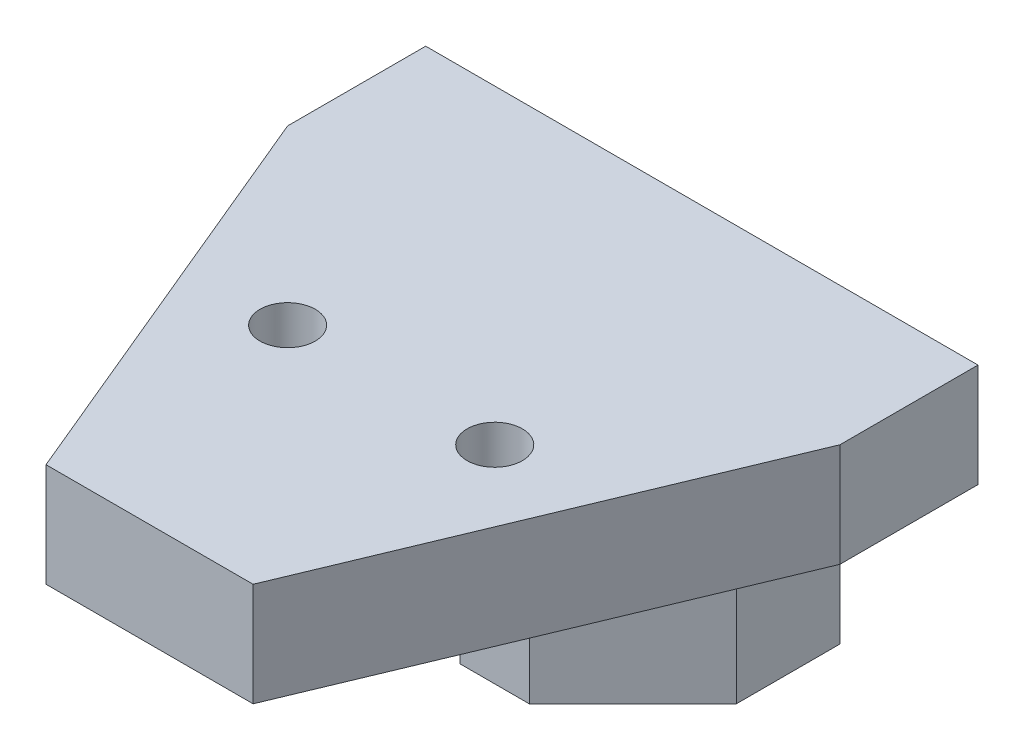
ISO-10303-21;
HEADER;
FILE_DESCRIPTION(('STEP AP214'),'2;1');
FILE_NAME('part.step','',(''),(''),'','','');
FILE_SCHEMA(('AUTOMOTIVE_DESIGN { 1 0 10303 214 1 1 1 1 }'));
ENDSEC;
DATA;
#1=APPLICATION_CONTEXT('core data for automotive mechanical design processes');
#2=APPLICATION_PROTOCOL_DEFINITION('international standard','automotive_design',2000,#1);
#3=PRODUCT_CONTEXT('',#1,'mechanical');
#4=PRODUCT('Part','Part','',(#3));
#5=PRODUCT_RELATED_PRODUCT_CATEGORY('part','',(#4));
#6=PRODUCT_DEFINITION_FORMATION('','',#4);
#7=PRODUCT_DEFINITION_CONTEXT('part definition',#1,'design');
#8=PRODUCT_DEFINITION('design','',#6,#7);
#9=PRODUCT_DEFINITION_SHAPE('','',#8);
#10=(LENGTH_UNIT() NAMED_UNIT(*) SI_UNIT(.MILLI.,.METRE.));
#11=(NAMED_UNIT(*) PLANE_ANGLE_UNIT() SI_UNIT($,.RADIAN.));
#12=(NAMED_UNIT(*) SI_UNIT($,.STERADIAN.) SOLID_ANGLE_UNIT());
#13=UNCERTAINTY_MEASURE_WITH_UNIT(LENGTH_MEASURE(1.E-05),#10,'distance_accuracy_value','');
#14=(GEOMETRIC_REPRESENTATION_CONTEXT(3) GLOBAL_UNCERTAINTY_ASSIGNED_CONTEXT((#13)) GLOBAL_UNIT_ASSIGNED_CONTEXT((#10,
#11,#12)) REPRESENTATION_CONTEXT('',''));
#15=CARTESIAN_POINT('',(0.,0.,0.));
#16=DIRECTION('',(0.,0.,1.));
#17=DIRECTION('',(1.,0.,0.));
#18=AXIS2_PLACEMENT_3D('',#15,#16,#17);
#19=CARTESIAN_POINT('',(0.,0.,20.));
#20=DIRECTION('',(0.,1.,0.));
#21=DIRECTION('',(0.,0.,1.));
#22=AXIS2_PLACEMENT_3D('',#19,#20,#21);
#23=PLANE('',#22);
#24=CARTESIAN_POINT('',(25.,0.,45.));
#25=DIRECTION('',(0.,-1.,0.));
#26=DIRECTION('',(0.,0.,-1.));
#27=AXIS2_PLACEMENT_3D('',#24,#25,#26);
#28=CIRCLE('',#27,4.);
#29=CARTESIAN_POINT('',(25.,0.,41.));
#30=VERTEX_POINT('',#29);
#31=EDGE_CURVE('E304',#30,#30,#28,.T.);
#32=ORIENTED_EDGE('',*,*,#31,.F.);
#33=EDGE_LOOP('',(#32));
#34=FACE_BOUND('',#33,.T.);
#35=CARTESIAN_POINT('',(55.,0.,45.));
#36=DIRECTION('',(0.,-1.,0.));
#37=DIRECTION('',(0.,0.,-1.));
#38=AXIS2_PLACEMENT_3D('',#35,#36,#37);
#39=CIRCLE('',#38,4.);
#40=CARTESIAN_POINT('',(55.,0.,41.));
#41=VERTEX_POINT('',#40);
#42=EDGE_CURVE('E305',#41,#41,#39,.T.);
#43=ORIENTED_EDGE('',*,*,#42,.F.);
#44=EDGE_LOOP('',(#43));
#45=FACE_BOUND('',#44,.T.);
#46=DIRECTION('',(0.,0.,-1.));
#47=VECTOR('',#46,1.);
#48=CARTESIAN_POINT('',(20.,0.,0.));
#49=LINE('',#48,#47);
#50=CARTESIAN_POINT('',(20.,0.,15.));
#51=VERTEX_POINT('',#50);
#52=CARTESIAN_POINT('',(20.,0.,0.));
#53=VERTEX_POINT('',#52);
#54=EDGE_CURVE('E58',#51,#53,#49,.T.);
#55=ORIENTED_EDGE('',*,*,#54,.F.);
#56=DIRECTION('',(-0.707106781186548,0.,-0.707106781186547));
#57=VECTOR('',#56,1.);
#58=CARTESIAN_POINT('',(35.,0.,30.));
#59=LINE('',#58,#57);
#60=CARTESIAN_POINT('',(35.,0.,30.));
#61=VERTEX_POINT('',#60);
#62=EDGE_CURVE('E64',#61,#51,#59,.T.);
#63=ORIENTED_EDGE('',*,*,#62,.F.);
#64=DIRECTION('',(-1.,0.,0.));
#65=VECTOR('',#64,1.);
#66=CARTESIAN_POINT('',(40.,0.,30.));
#67=LINE('',#66,#65);
#68=CARTESIAN_POINT('',(45.,0.,30.));
#69=VERTEX_POINT('',#68);
#70=EDGE_CURVE('E174',#69,#61,#67,.T.);
#71=ORIENTED_EDGE('',*,*,#70,.F.);
#72=DIRECTION('',(-0.707106781186547,0.,0.707106781186547));
#73=VECTOR('',#72,1.);
#74=CARTESIAN_POINT('',(45.,0.,30.));
#75=LINE('',#74,#73);
#76=CARTESIAN_POINT('',(60.,0.,15.));
#77=VERTEX_POINT('',#76);
#78=EDGE_CURVE('E168',#77,#69,#75,.T.);
#79=ORIENTED_EDGE('',*,*,#78,.F.);
#80=DIRECTION('',(0.,0.,1.));
#81=VECTOR('',#80,1.);
#82=CARTESIAN_POINT('',(60.,0.,0.));
#83=LINE('',#82,#81);
#84=CARTESIAN_POINT('',(60.,0.,0.));
#85=VERTEX_POINT('',#84);
#86=EDGE_CURVE('E169',#85,#77,#83,.T.);
#87=ORIENTED_EDGE('',*,*,#86,.F.);
#88=DIRECTION('',(1.,0.,0.));
#89=VECTOR('',#88,1.);
#90=CARTESIAN_POINT('',(0.,0.,0.));
#91=LINE('',#90,#89);
#92=CARTESIAN_POINT('',(80.,0.,0.));
#93=VERTEX_POINT('',#92);
#94=EDGE_CURVE('E146',#85,#93,#91,.T.);
#95=ORIENTED_EDGE('',*,*,#94,.T.);
#96=DIRECTION('',(0.,0.,-1.));
#97=VECTOR('',#96,1.);
#98=CARTESIAN_POINT('',(80.,0.,20.));
#99=LINE('',#98,#97);
#100=CARTESIAN_POINT('',(80.,0.,20.));
#101=VERTEX_POINT('',#100);
#102=EDGE_CURVE('E52',#101,#93,#99,.T.);
#103=ORIENTED_EDGE('',*,*,#102,.F.);
#104=DIRECTION('',(-0.384615384615385,0.,0.923076923076923));
#105=VECTOR('',#104,1.);
#106=CARTESIAN_POINT('',(55.,0.,80.));
#107=LINE('',#106,#105);
#108=CARTESIAN_POINT('',(55.,0.,80.));
#109=VERTEX_POINT('',#108);
#110=EDGE_CURVE('E203',#101,#109,#107,.T.);
#111=ORIENTED_EDGE('',*,*,#110,.T.);
#112=DIRECTION('',(-1.,0.,0.));
#113=VECTOR('',#112,1.);
#114=CARTESIAN_POINT('',(40.,0.,80.));
#115=LINE('',#114,#113);
#116=CARTESIAN_POINT('',(25.,0.,80.));
#117=VERTEX_POINT('',#116);
#118=EDGE_CURVE('E193',#109,#117,#115,.T.);
#119=ORIENTED_EDGE('',*,*,#118,.T.);
#120=DIRECTION('',(-0.384615384615385,0.,-0.923076923076923));
#121=VECTOR('',#120,1.);
#122=CARTESIAN_POINT('',(0.,0.,20.));
#123=LINE('',#122,#121);
#124=CARTESIAN_POINT('',(0.,0.,20.));
#125=VERTEX_POINT('',#124);
#126=EDGE_CURVE('E209',#117,#125,#123,.T.);
#127=ORIENTED_EDGE('',*,*,#126,.T.);
#128=DIRECTION('',(0.,0.,-1.));
#129=VECTOR('',#128,1.);
#130=CARTESIAN_POINT('',(0.,0.,20.));
#131=LINE('',#130,#129);
#132=CARTESIAN_POINT('',(0.,0.,0.));
#133=VERTEX_POINT('',#132);
#134=EDGE_CURVE('E11',#125,#133,#131,.T.);
#135=ORIENTED_EDGE('',*,*,#134,.T.);
#136=EDGE_CURVE('E226',#133,#53,#91,.T.);
#137=ORIENTED_EDGE('',*,*,#136,.T.);
#138=EDGE_LOOP('',(#55,#63,#71,#79,#87,#95,#103,#111,#119,#127,#135,#137));
#139=FACE_BOUND('',#138,.T.);
#140=ADVANCED_FACE('F44',(#34,#45,#139),#23,.F.);
#141=CARTESIAN_POINT('',(0.,10.,20.));
#142=DIRECTION('',(1.,0.,0.));
#143=DIRECTION('',(0.,0.,-1.));
#144=AXIS2_PLACEMENT_3D('',#141,#142,#143);
#145=PLANE('',#144);
#146=DIRECTION('',(0.,-1.,0.));
#147=VECTOR('',#146,1.);
#148=CARTESIAN_POINT('',(0.,10.,0.));
#149=LINE('',#148,#147);
#150=CARTESIAN_POINT('',(0.,15.,0.));
#151=VERTEX_POINT('',#150);
#152=EDGE_CURVE('E217',#151,#133,#149,.T.);
#153=ORIENTED_EDGE('',*,*,#152,.T.);
#154=ORIENTED_EDGE('',*,*,#134,.F.);
#155=DIRECTION('',(0.,-1.,0.));
#156=VECTOR('',#155,1.);
#157=CARTESIAN_POINT('',(0.,10.,20.));
#158=LINE('',#157,#156);
#159=CARTESIAN_POINT('',(0.,15.,20.));
#160=VERTEX_POINT('',#159);
#161=EDGE_CURVE('E219',#160,#125,#158,.T.);
#162=ORIENTED_EDGE('',*,*,#161,.F.);
#163=DIRECTION('',(0.,0.,-1.));
#164=VECTOR('',#163,1.);
#165=CARTESIAN_POINT('',(0.,15.,20.));
#166=LINE('',#165,#164);
#167=EDGE_CURVE('E192',#160,#151,#166,.T.);
#168=ORIENTED_EDGE('',*,*,#167,.T.);
#169=EDGE_LOOP('',(#153,#154,#162,#168));
#170=FACE_BOUND('',#169,.T.);
#171=ADVANCED_FACE('F50',(#170),#145,.F.);
#172=CARTESIAN_POINT('',(80.,0.,20.));
#173=DIRECTION('',(-1.,0.,0.));
#174=DIRECTION('',(0.,0.,1.));
#175=AXIS2_PLACEMENT_3D('',#172,#173,#174);
#176=PLANE('',#175);
#177=DIRECTION('',(0.,1.,0.));
#178=VECTOR('',#177,1.);
#179=CARTESIAN_POINT('',(80.,0.,0.));
#180=LINE('',#179,#178);
#181=CARTESIAN_POINT('',(80.,15.,0.));
#182=VERTEX_POINT('',#181);
#183=EDGE_CURVE('E221',#93,#182,#180,.T.);
#184=ORIENTED_EDGE('',*,*,#183,.T.);
#185=DIRECTION('',(0.,0.,-1.));
#186=VECTOR('',#185,1.);
#187=CARTESIAN_POINT('',(80.,15.,20.));
#188=LINE('',#187,#186);
#189=CARTESIAN_POINT('',(80.,15.,20.));
#190=VERTEX_POINT('',#189);
#191=EDGE_CURVE('E194',#190,#182,#188,.T.);
#192=ORIENTED_EDGE('',*,*,#191,.F.);
#193=DIRECTION('',(0.,1.,0.));
#194=VECTOR('',#193,1.);
#195=CARTESIAN_POINT('',(80.,0.,20.));
#196=LINE('',#195,#194);
#197=EDGE_CURVE('E224',#101,#190,#196,.T.);
#198=ORIENTED_EDGE('',*,*,#197,.F.);
#199=ORIENTED_EDGE('',*,*,#102,.T.);
#200=EDGE_LOOP('',(#184,#192,#198,#199));
#201=FACE_BOUND('',#200,.T.);
#202=ADVANCED_FACE('F235',(#201),#176,.F.);
#203=CARTESIAN_POINT('',(0.,0.,0.));
#204=DIRECTION('',(0.,0.,1.));
#205=DIRECTION('',(1.,0.,0.));
#206=AXIS2_PLACEMENT_3D('',#203,#204,#205);
#207=PLANE('',#206);
#208=ORIENTED_EDGE('',*,*,#152,.F.);
#209=DIRECTION('',(1.,0.,0.));
#210=VECTOR('',#209,1.);
#211=CARTESIAN_POINT('',(80.,15.,0.));
#212=LINE('',#211,#210);
#213=EDGE_CURVE('E151',#151,#182,#212,.T.);
#214=ORIENTED_EDGE('',*,*,#213,.T.);
#215=ORIENTED_EDGE('',*,*,#183,.F.);
#216=ORIENTED_EDGE('',*,*,#94,.F.);
#217=DIRECTION('',(0.,1.,0.));
#218=VECTOR('',#217,1.);
#219=CARTESIAN_POINT('',(60.,-30.,0.));
#220=LINE('',#219,#218);
#221=CARTESIAN_POINT('',(60.,-30.,0.));
#222=VERTEX_POINT('',#221);
#223=EDGE_CURVE('E144',#222,#85,#220,.T.);
#224=ORIENTED_EDGE('',*,*,#223,.F.);
#225=DIRECTION('',(1.,0.,0.));
#226=VECTOR('',#225,1.);
#227=CARTESIAN_POINT('',(40.,-30.,0.));
#228=LINE('',#227,#226);
#229=CARTESIAN_POINT('',(20.,-30.,0.));
#230=VERTEX_POINT('',#229);
#231=EDGE_CURVE('E133',#230,#222,#228,.T.);
#232=ORIENTED_EDGE('',*,*,#231,.F.);
#233=DIRECTION('',(0.,1.,0.));
#234=VECTOR('',#233,1.);
#235=CARTESIAN_POINT('',(20.,-30.,0.));
#236=LINE('',#235,#234);
#237=EDGE_CURVE('E170',#230,#53,#236,.T.);
#238=ORIENTED_EDGE('',*,*,#237,.T.);
#239=ORIENTED_EDGE('',*,*,#136,.F.);
#240=EDGE_LOOP('',(#208,#214,#215,#216,#224,#232,#238,#239));
#241=FACE_BOUND('',#240,.T.);
#242=ADVANCED_FACE('F148',(#241),#207,.F.);
#243=CARTESIAN_POINT('',(55.,15.,80.));
#244=DIRECTION('',(0.923076923076923,0.,0.384615384615385));
#245=DIRECTION('',(0.384615384615385,0.,-0.923076923076923));
#246=AXIS2_PLACEMENT_3D('',#243,#244,#245);
#247=PLANE('',#246);
#248=ORIENTED_EDGE('',*,*,#110,.F.);
#249=ORIENTED_EDGE('',*,*,#197,.T.);
#250=DIRECTION('',(-0.384615384615385,0.,0.923076923076923));
#251=VECTOR('',#250,1.);
#252=CARTESIAN_POINT('',(55.,15.,80.));
#253=LINE('',#252,#251);
#254=CARTESIAN_POINT('',(55.,15.,80.));
#255=VERTEX_POINT('',#254);
#256=EDGE_CURVE('E204',#190,#255,#253,.T.);
#257=ORIENTED_EDGE('',*,*,#256,.T.);
#258=DIRECTION('',(0.,-1.,0.));
#259=VECTOR('',#258,1.);
#260=CARTESIAN_POINT('',(55.,15.,80.));
#261=LINE('',#260,#259);
#262=EDGE_CURVE('E214',#255,#109,#261,.T.);
#263=ORIENTED_EDGE('',*,*,#262,.T.);
#264=EDGE_LOOP('',(#248,#249,#257,#263));
#265=FACE_BOUND('',#264,.T.);
#266=ADVANCED_FACE('F244',(#265),#247,.T.);
#267=CARTESIAN_POINT('',(0.,15.,20.));
#268=DIRECTION('',(-0.923076923076923,0.,0.384615384615385));
#269=DIRECTION('',(0.384615384615385,0.,0.923076923076923));
#270=AXIS2_PLACEMENT_3D('',#267,#268,#269);
#271=PLANE('',#270);
#272=ORIENTED_EDGE('',*,*,#126,.F.);
#273=DIRECTION('',(0.,-1.,0.));
#274=VECTOR('',#273,1.);
#275=CARTESIAN_POINT('',(25.,15.,80.));
#276=LINE('',#275,#274);
#277=CARTESIAN_POINT('',(25.,15.,80.));
#278=VERTEX_POINT('',#277);
#279=EDGE_CURVE('E210',#278,#117,#276,.T.);
#280=ORIENTED_EDGE('',*,*,#279,.F.);
#281=DIRECTION('',(-0.384615384615385,0.,-0.923076923076923));
#282=VECTOR('',#281,1.);
#283=CARTESIAN_POINT('',(0.,15.,20.));
#284=LINE('',#283,#282);
#285=EDGE_CURVE('E199',#278,#160,#284,.T.);
#286=ORIENTED_EDGE('',*,*,#285,.T.);
#287=ORIENTED_EDGE('',*,*,#161,.T.);
#288=EDGE_LOOP('',(#272,#280,#286,#287));
#289=FACE_BOUND('',#288,.T.);
#290=ADVANCED_FACE('F248',(#289),#271,.T.);
#291=CARTESIAN_POINT('',(40.,15.,80.));
#292=DIRECTION('',(0.,0.,1.));
#293=DIRECTION('',(1.,0.,0.));
#294=AXIS2_PLACEMENT_3D('',#291,#292,#293);
#295=PLANE('',#294);
#296=ORIENTED_EDGE('',*,*,#118,.F.);
#297=ORIENTED_EDGE('',*,*,#262,.F.);
#298=DIRECTION('',(-1.,0.,0.));
#299=VECTOR('',#298,1.);
#300=CARTESIAN_POINT('',(40.,15.,80.));
#301=LINE('',#300,#299);
#302=EDGE_CURVE('E196',#255,#278,#301,.T.);
#303=ORIENTED_EDGE('',*,*,#302,.T.);
#304=ORIENTED_EDGE('',*,*,#279,.T.);
#305=EDGE_LOOP('',(#296,#297,#303,#304));
#306=FACE_BOUND('',#305,.T.);
#307=ADVANCED_FACE('F249',(#306),#295,.T.);
#308=CARTESIAN_POINT('',(0.,15.,0.));
#309=DIRECTION('',(0.,1.,0.));
#310=DIRECTION('',(0.,0.,1.));
#311=AXIS2_PLACEMENT_3D('',#308,#309,#310);
#312=PLANE('',#311);
#313=CARTESIAN_POINT('',(25.,15.,45.));
#314=DIRECTION('',(0.,-1.,0.));
#315=DIRECTION('',(0.,0.,-1.));
#316=AXIS2_PLACEMENT_3D('',#313,#314,#315);
#317=CIRCLE('',#316,4.);
#318=CARTESIAN_POINT('',(25.,15.,41.));
#319=VERTEX_POINT('',#318);
#320=EDGE_CURVE('E173',#319,#319,#317,.T.);
#321=ORIENTED_EDGE('',*,*,#320,.T.);
#322=EDGE_LOOP('',(#321));
#323=FACE_BOUND('',#322,.T.);
#324=CARTESIAN_POINT('',(55.,15.,45.));
#325=DIRECTION('',(0.,-1.,0.));
#326=DIRECTION('',(0.,0.,-1.));
#327=AXIS2_PLACEMENT_3D('',#324,#325,#326);
#328=CIRCLE('',#327,4.);
#329=CARTESIAN_POINT('',(55.,15.,41.));
#330=VERTEX_POINT('',#329);
#331=EDGE_CURVE('E297',#330,#330,#328,.T.);
#332=ORIENTED_EDGE('',*,*,#331,.T.);
#333=EDGE_LOOP('',(#332));
#334=FACE_BOUND('',#333,.T.);
#335=ORIENTED_EDGE('',*,*,#302,.F.);
#336=ORIENTED_EDGE('',*,*,#256,.F.);
#337=ORIENTED_EDGE('',*,*,#191,.T.);
#338=ORIENTED_EDGE('',*,*,#213,.F.);
#339=ORIENTED_EDGE('',*,*,#167,.F.);
#340=ORIENTED_EDGE('',*,*,#285,.F.);
#341=EDGE_LOOP('',(#335,#336,#337,#338,#339,#340));
#342=FACE_BOUND('',#341,.T.);
#343=ADVANCED_FACE('F238',(#323,#334,#342),#312,.T.);
#344=CARTESIAN_POINT('',(60.,-30.,0.));
#345=DIRECTION('',(-1.,0.,0.));
#346=DIRECTION('',(0.,0.,1.));
#347=AXIS2_PLACEMENT_3D('',#344,#345,#346);
#348=PLANE('',#347);
#349=ORIENTED_EDGE('',*,*,#86,.T.);
#350=DIRECTION('',(0.,1.,0.));
#351=VECTOR('',#350,1.);
#352=CARTESIAN_POINT('',(60.,-30.,15.));
#353=LINE('',#352,#351);
#354=CARTESIAN_POINT('',(60.,-30.,15.));
#355=VERTEX_POINT('',#354);
#356=EDGE_CURVE('E155',#355,#77,#353,.T.);
#357=ORIENTED_EDGE('',*,*,#356,.F.);
#358=DIRECTION('',(0.,0.,1.));
#359=VECTOR('',#358,1.);
#360=CARTESIAN_POINT('',(60.,-30.,0.));
#361=LINE('',#360,#359);
#362=EDGE_CURVE('E132',#222,#355,#361,.T.);
#363=ORIENTED_EDGE('',*,*,#362,.F.);
#364=ORIENTED_EDGE('',*,*,#223,.T.);
#365=EDGE_LOOP('',(#349,#357,#363,#364));
#366=FACE_BOUND('',#365,.T.);
#367=ADVANCED_FACE('F152',(#366),#348,.F.);
#368=CARTESIAN_POINT('',(45.,-30.,30.));
#369=DIRECTION('',(-0.707106781186547,0.,-0.707106781186547));
#370=DIRECTION('',(-0.707106781186548,0.,0.707106781186548));
#371=AXIS2_PLACEMENT_3D('',#368,#369,#370);
#372=PLANE('',#371);
#373=ORIENTED_EDGE('',*,*,#78,.T.);
#374=DIRECTION('',(0.,1.,0.));
#375=VECTOR('',#374,1.);
#376=CARTESIAN_POINT('',(45.,-30.,30.));
#377=LINE('',#376,#375);
#378=CARTESIAN_POINT('',(45.,-30.,30.));
#379=VERTEX_POINT('',#378);
#380=EDGE_CURVE('E183',#379,#69,#377,.T.);
#381=ORIENTED_EDGE('',*,*,#380,.F.);
#382=DIRECTION('',(-0.707106781186547,0.,0.707106781186547));
#383=VECTOR('',#382,1.);
#384=CARTESIAN_POINT('',(45.,-30.,30.));
#385=LINE('',#384,#383);
#386=EDGE_CURVE('E160',#355,#379,#385,.T.);
#387=ORIENTED_EDGE('',*,*,#386,.F.);
#388=ORIENTED_EDGE('',*,*,#356,.T.);
#389=EDGE_LOOP('',(#373,#381,#387,#388));
#390=FACE_BOUND('',#389,.T.);
#391=ADVANCED_FACE('F262',(#390),#372,.F.);
#392=CARTESIAN_POINT('',(40.,-30.,30.));
#393=DIRECTION('',(0.,0.,-1.));
#394=DIRECTION('',(-1.,0.,0.));
#395=AXIS2_PLACEMENT_3D('',#392,#393,#394);
#396=PLANE('',#395);
#397=ORIENTED_EDGE('',*,*,#70,.T.);
#398=DIRECTION('',(0.,1.,0.));
#399=VECTOR('',#398,1.);
#400=CARTESIAN_POINT('',(35.,-30.,30.));
#401=LINE('',#400,#399);
#402=CARTESIAN_POINT('',(35.,-30.,30.));
#403=VERTEX_POINT('',#402);
#404=EDGE_CURVE('E185',#403,#61,#401,.T.);
#405=ORIENTED_EDGE('',*,*,#404,.F.);
#406=DIRECTION('',(-1.,0.,0.));
#407=VECTOR('',#406,1.);
#408=CARTESIAN_POINT('',(40.,-30.,30.));
#409=LINE('',#408,#407);
#410=EDGE_CURVE('E157',#379,#403,#409,.T.);
#411=ORIENTED_EDGE('',*,*,#410,.F.);
#412=ORIENTED_EDGE('',*,*,#380,.T.);
#413=EDGE_LOOP('',(#397,#405,#411,#412));
#414=FACE_BOUND('',#413,.T.);
#415=ADVANCED_FACE('F261',(#414),#396,.F.);
#416=CARTESIAN_POINT('',(35.,-30.,30.));
#417=DIRECTION('',(0.707106781186547,0.,-0.707106781186548));
#418=DIRECTION('',(-0.707106781186548,0.,-0.707106781186547));
#419=AXIS2_PLACEMENT_3D('',#416,#417,#418);
#420=PLANE('',#419);
#421=ORIENTED_EDGE('',*,*,#62,.T.);
#422=DIRECTION('',(0.,1.,0.));
#423=VECTOR('',#422,1.);
#424=CARTESIAN_POINT('',(20.,-30.,15.));
#425=LINE('',#424,#423);
#426=CARTESIAN_POINT('',(20.,-30.,15.));
#427=VERTEX_POINT('',#426);
#428=EDGE_CURVE('E176',#427,#51,#425,.T.);
#429=ORIENTED_EDGE('',*,*,#428,.F.);
#430=DIRECTION('',(-0.707106781186548,0.,-0.707106781186547));
#431=VECTOR('',#430,1.);
#432=CARTESIAN_POINT('',(35.,-30.,30.));
#433=LINE('',#432,#431);
#434=EDGE_CURVE('E163',#403,#427,#433,.T.);
#435=ORIENTED_EDGE('',*,*,#434,.F.);
#436=ORIENTED_EDGE('',*,*,#404,.T.);
#437=EDGE_LOOP('',(#421,#429,#435,#436));
#438=FACE_BOUND('',#437,.T.);
#439=ADVANCED_FACE('F260',(#438),#420,.F.);
#440=CARTESIAN_POINT('',(20.,-30.,0.));
#441=DIRECTION('',(1.,0.,0.));
#442=DIRECTION('',(0.,0.,-1.));
#443=AXIS2_PLACEMENT_3D('',#440,#441,#442);
#444=PLANE('',#443);
#445=ORIENTED_EDGE('',*,*,#54,.T.);
#446=ORIENTED_EDGE('',*,*,#237,.F.);
#447=DIRECTION('',(0.,0.,-1.));
#448=VECTOR('',#447,1.);
#449=CARTESIAN_POINT('',(20.,-30.,0.));
#450=LINE('',#449,#448);
#451=EDGE_CURVE('E140',#427,#230,#450,.T.);
#452=ORIENTED_EDGE('',*,*,#451,.F.);
#453=ORIENTED_EDGE('',*,*,#428,.T.);
#454=EDGE_LOOP('',(#445,#446,#452,#453));
#455=FACE_BOUND('',#454,.T.);
#456=ADVANCED_FACE('F251',(#455),#444,.F.);
#457=CARTESIAN_POINT('',(0.,-30.,0.));
#458=DIRECTION('',(0.,1.,0.));
#459=DIRECTION('',(0.,0.,1.));
#460=AXIS2_PLACEMENT_3D('',#457,#458,#459);
#461=PLANE('',#460);
#462=ORIENTED_EDGE('',*,*,#231,.T.);
#463=ORIENTED_EDGE('',*,*,#362,.T.);
#464=ORIENTED_EDGE('',*,*,#386,.T.);
#465=ORIENTED_EDGE('',*,*,#410,.T.);
#466=ORIENTED_EDGE('',*,*,#434,.T.);
#467=ORIENTED_EDGE('',*,*,#451,.T.);
#468=EDGE_LOOP('',(#462,#463,#464,#465,#466,#467));
#469=FACE_BOUND('',#468,.T.);
#470=ADVANCED_FACE('F131',(#469),#461,.F.);
#471=CARTESIAN_POINT('',(55.,15.,45.));
#472=DIRECTION('',(0.,-1.,0.));
#473=DIRECTION('',(0.,0.,-1.));
#474=AXIS2_PLACEMENT_3D('',#471,#472,#473);
#475=CYLINDRICAL_SURFACE('',#474,4.);
#476=ORIENTED_EDGE('',*,*,#331,.F.);
#477=EDGE_LOOP('',(#476));
#478=FACE_BOUND('',#477,.T.);
#479=ORIENTED_EDGE('',*,*,#42,.T.);
#480=EDGE_LOOP('',(#479));
#481=FACE_BOUND('',#480,.T.);
#482=ADVANCED_FACE('F313',(#478,#481),#475,.F.);
#483=CARTESIAN_POINT('',(25.,15.,45.));
#484=DIRECTION('',(0.,-1.,0.));
#485=DIRECTION('',(0.,0.,-1.));
#486=AXIS2_PLACEMENT_3D('',#483,#484,#485);
#487=CYLINDRICAL_SURFACE('',#486,4.);
#488=ORIENTED_EDGE('',*,*,#320,.F.);
#489=EDGE_LOOP('',(#488));
#490=FACE_BOUND('',#489,.T.);
#491=ORIENTED_EDGE('',*,*,#31,.T.);
#492=EDGE_LOOP('',(#491));
#493=FACE_BOUND('',#492,.T.);
#494=ADVANCED_FACE('F311',(#490,#493),#487,.F.);
#495=CLOSED_SHELL('',(#140,#171,#202,#242,#266,#290,#307,#343,#367,#391,#415,#439,#456,#470,
#482,#494));
#496=MANIFOLD_SOLID_BREP('B2',#495);
#497=ADVANCED_BREP_SHAPE_REPRESENTATION('',(#18,#496),#14);
#498=SHAPE_DEFINITION_REPRESENTATION(#9,#497);
ENDSEC;
END-ISO-10303-21;
